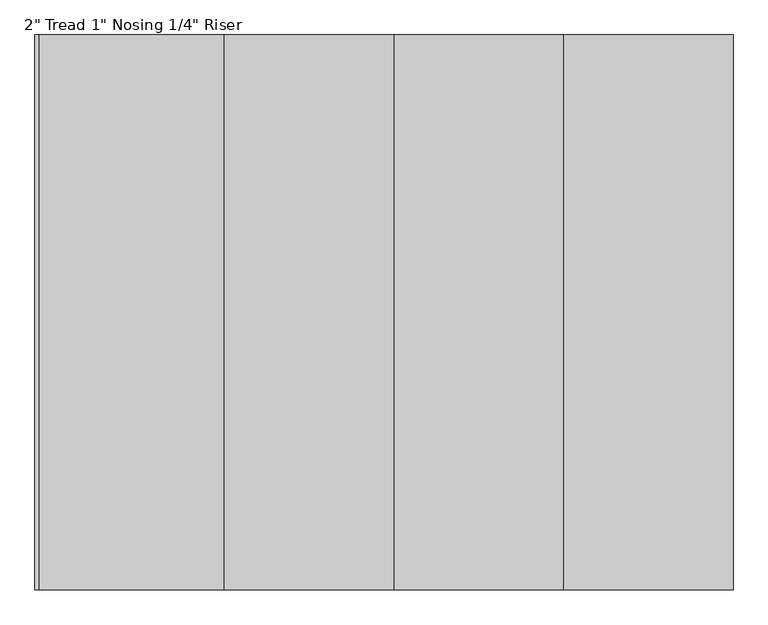
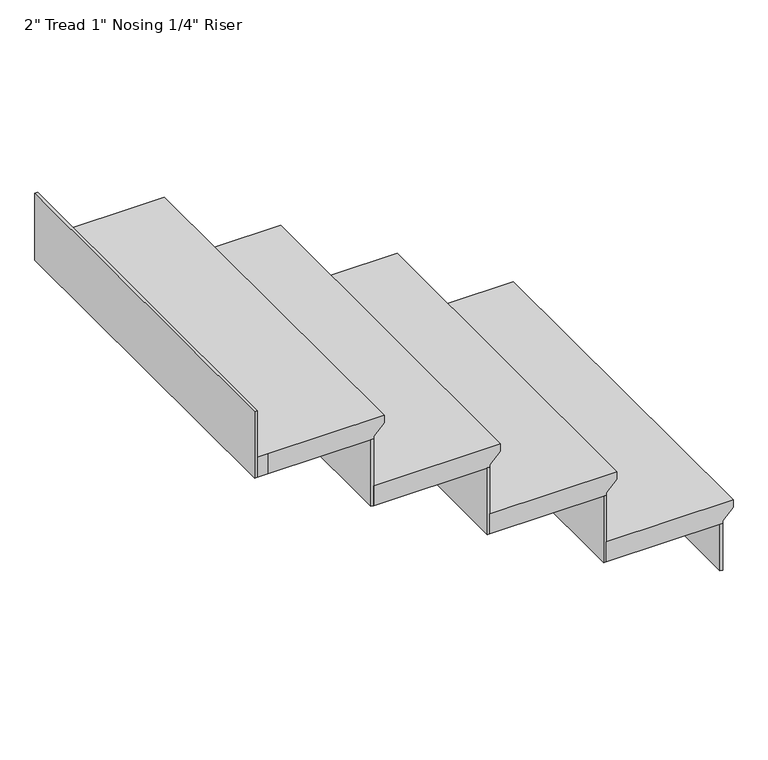
"""IFC4 building model written with IfcOpenShell, lengths in millimetres: stair flight geometry."""

from ifc_helpers import new_model, si_unit, origin, place, context, project, spatial, faceted_brep, source, transform, mapped, element, save


def stair_flight_2df9e6b5(model_context):
    return source(origin(), model_context, "Body", "Brep", [
        faceted_brep([(5470.6597674, -1392.6241735, 319.6166667), (5470.6597674, -1392.6241735, 338.6666667), (5470.6597674, -2307.0241735, 338.6666667), (5470.6597674, -2307.0241735, 319.6166667), (5445.2597674, -1392.6241735, 294.2166667), (5445.2597674, -2307.0241735, 294.2166667), (5165.8597674, -1392.6241735, 338.6666667), (5165.8597674, -2307.0241735, 338.6666667), (5445.2597674, -2307.0241735, 287.8666667), (5165.8597674, -2307.0241735, 287.8666667), (5165.8597674, -1392.6241735, 287.8666667), (5445.2597674, -1392.6241735, 287.8666667)], [[[0, 1, 2, 3]], [[4, 0, 3, 5]], [[2, 1, 6, 7]], [[8, 9, 10, 11]], [[2, 7, 9, 8, 5, 3]], [[8, 11, 4, 5]], [[6, 1, 0, 4, 11, 10]], [[7, 6, 10, 9]]]),
        faceted_brep([(5445.2597674, -1392.6241735, 287.8666667), (5445.2597674, -1392.6241735, 169.3333333), (5438.9097674, -1392.6241735, 169.3333333), (5438.9097674, -1392.6241735, 287.8666667), (5445.2597674, -2307.0241735, 287.8666667), (5438.9097674, -2307.0241735, 287.8666667), (5438.9097674, -2307.0241735, 169.3333333), (5445.2597674, -2307.0241735, 169.3333333)], [[[0, 1, 2, 3]], [[4, 5, 6, 7]], [[1, 0, 4, 7]], [[2, 1, 7, 6]], [[3, 2, 6, 5]], [[0, 3, 5, 4]]]),
        faceted_brep([(5165.8597674, -1392.6241735, 457.2), (5165.8597674, -1392.6241735, 287.8666667), (5159.5097674, -1392.6241735, 287.8666667), (5159.5097674, -1392.6241735, 457.2), (5165.8597674, -2307.0241735, 457.2), (5159.5097674, -2307.0241735, 457.2), (5159.5097674, -2307.0241735, 287.8666667), (5165.8597674, -2307.0241735, 287.8666667)], [[[0, 1, 2, 3]], [[4, 5, 6, 7]], [[1, 0, 4, 7]], [[2, 1, 7, 6]], [[3, 2, 6, 5]], [[0, 3, 5, 4]]]),
        faceted_brep([(5191.2597674, -2307.0241735, 508.0), (5191.2597674, -1392.6241735, 508.0), (4886.4597674, -1392.6241735, 508.0), (4886.4597674, -2307.0241735, 508.0), (5165.8597674, -2307.0241735, 457.2), (4886.4597674, -2307.0241735, 457.2), (4886.4597674, -1392.6241735, 457.2), (5165.8597674, -1392.6241735, 457.2), (5165.8597674, -2307.0241735, 463.55), (5191.2597674, -2307.0241735, 488.95), (5165.8597674, -1392.6241735, 463.55), (5191.2597674, -1392.6241735, 488.95)], [[[0, 1, 2, 3]], [[4, 5, 6, 7]], [[0, 3, 5, 4, 8, 9]], [[4, 7, 10, 8]], [[2, 1, 11, 10, 7, 6]], [[3, 2, 6, 5]], [[11, 1, 0, 9]], [[10, 11, 9, 8]]]),
        faceted_brep([(4886.4597674, -1392.6241735, 626.5333333), (4886.4597674, -1392.6241735, 457.2), (4880.1097674, -1392.6241735, 457.2), (4880.1097674, -1392.6241735, 626.5333333), (4886.4597674, -2307.0241735, 626.5333333), (4880.1097674, -2307.0241735, 626.5333333), (4880.1097674, -2307.0241735, 457.2), (4886.4597674, -2307.0241735, 457.2)], [[[0, 1, 2, 3]], [[4, 5, 6, 7]], [[1, 0, 4, 7]], [[2, 1, 7, 6]], [[3, 2, 6, 5]], [[0, 3, 5, 4]]]),
        faceted_brep([(4911.8597674, -2307.0241735, 677.3333333), (4911.8597674, -1392.6241735, 677.3333333), (4607.0597674, -1392.6241735, 677.3333333), (4607.0597674, -2307.0241735, 677.3333333), (4886.4597674, -2307.0241735, 626.5333333), (4607.0597674, -2307.0241735, 626.5333333), (4607.0597674, -1392.6241735, 626.5333333), (4886.4597674, -1392.6241735, 626.5333333), (4886.4597674, -2307.0241735, 632.8833333), (4911.8597674, -2307.0241735, 658.2833333), (4886.4597674, -1392.6241735, 632.8833333), (4911.8597674, -1392.6241735, 658.2833333)], [[[0, 1, 2, 3]], [[4, 5, 6, 7]], [[0, 3, 5, 4, 8, 9]], [[4, 7, 10, 8]], [[2, 1, 11, 10, 7, 6]], [[3, 2, 6, 5]], [[11, 1, 0, 9]], [[10, 11, 9, 8]]]),
        faceted_brep([(4607.0597674, -1392.6241735, 795.8666667), (4607.0597674, -1392.6241735, 626.5333333), (4600.7097674, -1392.6241735, 626.5333333), (4600.7097674, -1392.6241735, 795.8666667), (4607.0597674, -2307.0241735, 795.8666667), (4600.7097674, -2307.0241735, 795.8666667), (4600.7097674, -2307.0241735, 626.5333333), (4607.0597674, -2307.0241735, 626.5333333)], [[[0, 1, 2, 3]], [[4, 5, 6, 7]], [[1, 0, 4, 7]], [[2, 1, 7, 6]], [[3, 2, 6, 5]], [[0, 3, 5, 4]]]),
        faceted_brep([(4327.6597674, -1392.6241735, 965.2), (4327.6597674, -1392.6241735, 795.8666667), (4321.3097674, -1392.6241735, 795.8666667), (4321.3097674, -1392.6241735, 965.2), (4327.6597674, -2307.0241735, 965.2), (4321.3097674, -2307.0241735, 965.2), (4321.3097674, -2307.0241735, 795.8666667), (4327.6597674, -2307.0241735, 795.8666667)], [[[0, 1, 2, 3]], [[4, 5, 6, 7]], [[1, 0, 4, 7]], [[2, 1, 7, 6]], [[3, 2, 6, 5]], [[0, 3, 5, 4]]]),
        faceted_brep([(4327.6597674, -2307.0241735, 846.6666667), (4353.0597674, -2307.0241735, 846.6666667), (4632.4597674, -2307.0241735, 846.6666667), (4632.4597674, -1392.6241735, 846.6666667), (4327.6597674, -1392.6241735, 846.6666667), (4353.0597674, -2307.0241735, 795.8666667), (4327.6597674, -2307.0241735, 795.8666667), (4327.6597674, -1392.6241735, 795.8666667), (4607.0597674, -1392.6241735, 795.8666667), (4607.0597674, -2307.0241735, 795.8666667), (4607.0597674, -2307.0241735, 802.2166667), (4632.4597674, -2307.0241735, 827.6166667), (4607.0597674, -1392.6241735, 802.2166667), (4632.4597674, -1392.6241735, 827.6166667)], [[[0, 1, 2, 3, 4]], [[5, 6, 7, 8, 9]], [[1, 0, 6, 5]], [[2, 1, 5, 9, 10, 11]], [[9, 8, 12, 10]], [[4, 3, 13, 12, 8, 7]], [[0, 4, 7, 6]], [[13, 3, 2, 11]], [[12, 13, 11, 10]]]),
    ])


if __name__ == "__main__":
    model = new_model("IFC4")
    model_context = context("Model", 3, world=origin())
    ifc_project = project(units=[si_unit("LENGTHUNIT", "METRE", prefix="MILLI")], contexts=[model_context])
    site = spatial("IfcSite", under=ifc_project)
    building = spatial("IfcBuilding", under=site)
    placement = place(None, origin())
    stair_flight_shape = stair_flight_2df9e6b5(model_context)
    element("IfcStairFlight", 1, ObjectType="2\" Tread 1\" Nosing 1/4\" Riser", at=placement, inside=building, context=model_context, shape_type="MappedRepresentation", body=[
        mapped(stair_flight_shape, transform((0.0, 0.0, 0.0), x_axis=(1.0, 0.0, 0.0), y_axis=(0.0, 1.0, 0.0), z_axis=(0.0, 0.0, 1.0))),
    ])
    save(model, "model.ifc")
